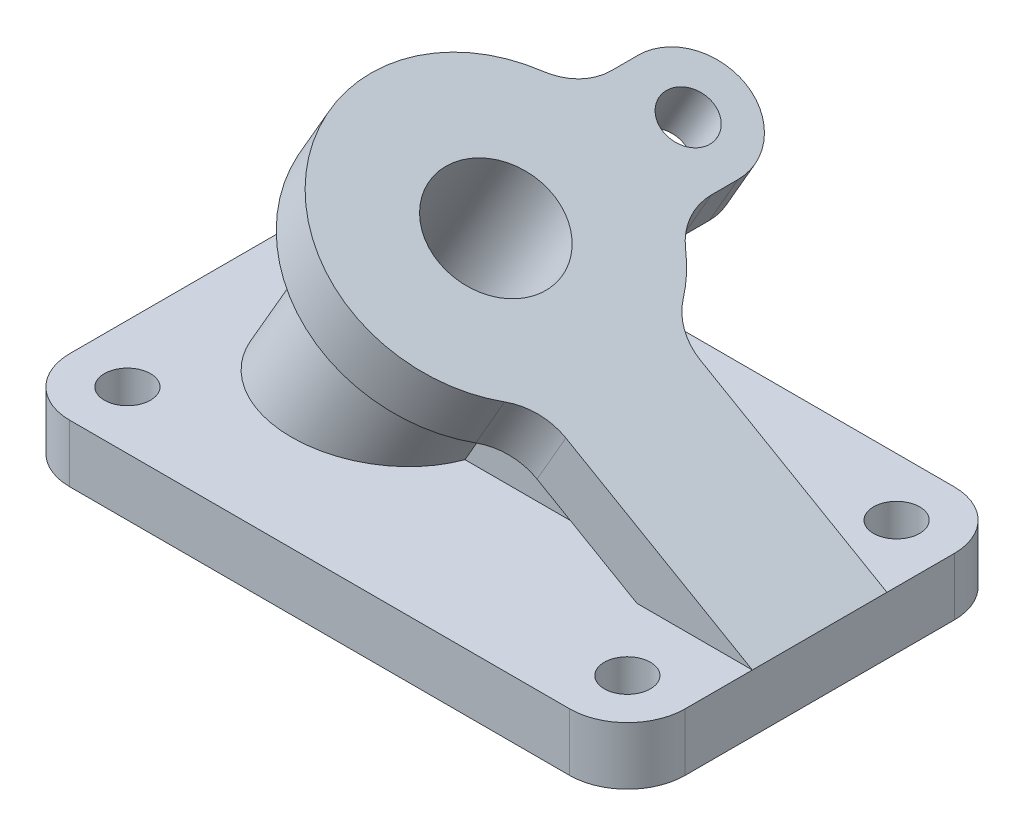
ISO-10303-21;
HEADER;
FILE_DESCRIPTION(('STEP AP214'),'2;1');
FILE_NAME('part.step','',(''),(''),'','','');
FILE_SCHEMA(('AUTOMOTIVE_DESIGN { 1 0 10303 214 1 1 1 1 }'));
ENDSEC;
DATA;
#1=APPLICATION_CONTEXT('core data for automotive mechanical design processes');
#2=APPLICATION_PROTOCOL_DEFINITION('international standard','automotive_design',2000,#1);
#3=PRODUCT_CONTEXT('',#1,'mechanical');
#4=PRODUCT('Part','Part','',(#3));
#5=PRODUCT_RELATED_PRODUCT_CATEGORY('part','',(#4));
#6=PRODUCT_DEFINITION_FORMATION('','',#4);
#7=PRODUCT_DEFINITION_CONTEXT('part definition',#1,'design');
#8=PRODUCT_DEFINITION('design','',#6,#7);
#9=PRODUCT_DEFINITION_SHAPE('','',#8);
#10=(LENGTH_UNIT() NAMED_UNIT(*) SI_UNIT(.MILLI.,.METRE.));
#11=(NAMED_UNIT(*) PLANE_ANGLE_UNIT() SI_UNIT($,.RADIAN.));
#12=(NAMED_UNIT(*) SI_UNIT($,.STERADIAN.) SOLID_ANGLE_UNIT());
#13=UNCERTAINTY_MEASURE_WITH_UNIT(LENGTH_MEASURE(1.E-05),#10,'distance_accuracy_value','');
#14=(GEOMETRIC_REPRESENTATION_CONTEXT(3) GLOBAL_UNCERTAINTY_ASSIGNED_CONTEXT((#13)) GLOBAL_UNIT_ASSIGNED_CONTEXT((#10,
#11,#12)) REPRESENTATION_CONTEXT('',''));
#15=CARTESIAN_POINT('',(0.,0.,0.));
#16=DIRECTION('',(0.,0.,1.));
#17=DIRECTION('',(1.,0.,0.));
#18=AXIS2_PLACEMENT_3D('',#15,#16,#17);
#19=CARTESIAN_POINT('',(0.,15.,0.));
#20=DIRECTION('',(0.,-1.,0.));
#21=DIRECTION('',(0.,0.,-1.));
#22=AXIS2_PLACEMENT_3D('',#19,#20,#21);
#23=PLANE('',#22);
#24=CARTESIAN_POINT('',(-65.,15.,-35.));
#25=DIRECTION('',(0.,1.,0.));
#26=DIRECTION('',(0.,0.,1.));
#27=AXIS2_PLACEMENT_3D('',#24,#25,#26);
#28=CIRCLE('',#27,6.);
#29=CARTESIAN_POINT('',(-65.,15.,-29.));
#30=VERTEX_POINT('',#29);
#31=EDGE_CURVE('E334',#30,#30,#28,.T.);
#32=ORIENTED_EDGE('',*,*,#31,.F.);
#33=EDGE_LOOP('',(#32));
#34=FACE_BOUND('',#33,.T.);
#35=CARTESIAN_POINT('',(65.,15.,-35.));
#36=DIRECTION('',(0.,1.,0.));
#37=DIRECTION('',(0.,0.,1.));
#38=AXIS2_PLACEMENT_3D('',#35,#36,#37);
#39=CIRCLE('',#38,6.);
#40=CARTESIAN_POINT('',(65.,15.,-29.));
#41=VERTEX_POINT('',#40);
#42=EDGE_CURVE('E329',#41,#41,#39,.T.);
#43=ORIENTED_EDGE('',*,*,#42,.F.);
#44=EDGE_LOOP('',(#43));
#45=FACE_BOUND('',#44,.T.);
#46=CARTESIAN_POINT('',(65.,15.,35.));
#47=DIRECTION('',(0.,1.,0.));
#48=DIRECTION('',(0.,0.,1.));
#49=AXIS2_PLACEMENT_3D('',#46,#47,#48);
#50=CIRCLE('',#49,6.);
#51=CARTESIAN_POINT('',(65.,15.,41.));
#52=VERTEX_POINT('',#51);
#53=EDGE_CURVE('E340',#52,#52,#50,.T.);
#54=ORIENTED_EDGE('',*,*,#53,.F.);
#55=EDGE_LOOP('',(#54));
#56=FACE_BOUND('',#55,.T.);
#57=CARTESIAN_POINT('',(-65.,15.,35.));
#58=DIRECTION('',(0.,1.,0.));
#59=DIRECTION('',(0.,0.,1.));
#60=AXIS2_PLACEMENT_3D('',#57,#58,#59);
#61=CIRCLE('',#60,6.);
#62=CARTESIAN_POINT('',(-65.,15.,41.));
#63=VERTEX_POINT('',#62);
#64=EDGE_CURVE('E344',#63,#63,#61,.T.);
#65=ORIENTED_EDGE('',*,*,#64,.F.);
#66=EDGE_LOOP('',(#65));
#67=FACE_BOUND('',#66,.T.);
#68=DIRECTION('',(0.,0.,1.));
#69=VECTOR('',#68,1.);
#70=CARTESIAN_POINT('',(49.9999999999997,15.,0.));
#71=LINE('',#70,#69);
#72=CARTESIAN_POINT('',(49.9999999999997,15.,-17.5));
#73=VERTEX_POINT('',#72);
#74=CARTESIAN_POINT('',(49.9999999999997,15.,-7.5));
#75=VERTEX_POINT('',#74);
#76=EDGE_CURVE('E309',#73,#75,#71,.T.);
#77=ORIENTED_EDGE('',*,*,#76,.F.);
#78=DIRECTION('',(1.,0.,0.));
#79=VECTOR('',#78,1.);
#80=CARTESIAN_POINT('',(0.,15.,-17.5));
#81=LINE('',#80,#79);
#82=CARTESIAN_POINT('',(80.,15.,-17.5));
#83=VERTEX_POINT('',#82);
#84=EDGE_CURVE('E11',#73,#83,#81,.T.);
#85=ORIENTED_EDGE('',*,*,#84,.T.);
#86=DIRECTION('',(0.,0.,-1.));
#87=VECTOR('',#86,1.);
#88=CARTESIAN_POINT('',(80.,15.,50.));
#89=LINE('',#88,#87);
#90=CARTESIAN_POINT('',(80.,15.,-35.));
#91=VERTEX_POINT('',#90);
#92=EDGE_CURVE('E360',#83,#91,#89,.T.);
#93=ORIENTED_EDGE('',*,*,#92,.T.);
#94=CARTESIAN_POINT('',(65.,15.,-35.));
#95=DIRECTION('',(0.,-1.,0.));
#96=DIRECTION('',(0.,0.,-1.));
#97=AXIS2_PLACEMENT_3D('',#94,#95,#96);
#98=CIRCLE('',#97,15.);
#99=CARTESIAN_POINT('',(65.,15.,-50.));
#100=VERTEX_POINT('',#99);
#101=EDGE_CURVE('E396',#91,#100,#98,.F.);
#102=ORIENTED_EDGE('',*,*,#101,.T.);
#103=DIRECTION('',(-1.,0.,0.));
#104=VECTOR('',#103,1.);
#105=CARTESIAN_POINT('',(-80.,15.,-50.));
#106=LINE('',#105,#104);
#107=CARTESIAN_POINT('',(-65.,15.,-50.));
#108=VERTEX_POINT('',#107);
#109=EDGE_CURVE('E357',#100,#108,#106,.T.);
#110=ORIENTED_EDGE('',*,*,#109,.T.);
#111=CARTESIAN_POINT('',(-65.,15.,-35.));
#112=DIRECTION('',(0.,-1.,0.));
#113=DIRECTION('',(0.,0.,-1.));
#114=AXIS2_PLACEMENT_3D('',#111,#112,#113);
#115=CIRCLE('',#114,15.);
#116=CARTESIAN_POINT('',(-80.,15.,-35.));
#117=VERTEX_POINT('',#116);
#118=EDGE_CURVE('E402',#108,#117,#115,.F.);
#119=ORIENTED_EDGE('',*,*,#118,.T.);
#120=DIRECTION('',(0.,0.,1.));
#121=VECTOR('',#120,1.);
#122=CARTESIAN_POINT('',(-80.,15.,50.));
#123=LINE('',#122,#121);
#124=CARTESIAN_POINT('',(-80.,15.,35.));
#125=VERTEX_POINT('',#124);
#126=EDGE_CURVE('E365',#117,#125,#123,.T.);
#127=ORIENTED_EDGE('',*,*,#126,.T.);
#128=CARTESIAN_POINT('',(-65.,15.,35.));
#129=DIRECTION('',(0.,-1.,0.));
#130=DIRECTION('',(0.,0.,-1.));
#131=AXIS2_PLACEMENT_3D('',#128,#129,#130);
#132=CIRCLE('',#131,15.);
#133=CARTESIAN_POINT('',(-65.,15.,50.));
#134=VERTEX_POINT('',#133);
#135=EDGE_CURVE('E394',#125,#134,#132,.F.);
#136=ORIENTED_EDGE('',*,*,#135,.T.);
#137=DIRECTION('',(1.,0.,0.));
#138=VECTOR('',#137,1.);
#139=CARTESIAN_POINT('',(-80.,15.,50.));
#140=LINE('',#139,#138);
#141=CARTESIAN_POINT('',(65.,15.,50.));
#142=VERTEX_POINT('',#141);
#143=EDGE_CURVE('E362',#134,#142,#140,.T.);
#144=ORIENTED_EDGE('',*,*,#143,.T.);
#145=CARTESIAN_POINT('',(65.,15.,35.));
#146=DIRECTION('',(0.,-1.,0.));
#147=DIRECTION('',(0.,0.,-1.));
#148=AXIS2_PLACEMENT_3D('',#145,#146,#147);
#149=CIRCLE('',#148,15.);
#150=CARTESIAN_POINT('',(80.,15.,35.));
#151=VERTEX_POINT('',#150);
#152=EDGE_CURVE('E400',#142,#151,#149,.F.);
#153=ORIENTED_EDGE('',*,*,#152,.T.);
#154=CARTESIAN_POINT('',(80.,15.,17.5));
#155=VERTEX_POINT('',#154);
#156=EDGE_CURVE('E351',#151,#155,#89,.T.);
#157=ORIENTED_EDGE('',*,*,#156,.T.);
#158=DIRECTION('',(1.,0.,0.));
#159=VECTOR('',#158,1.);
#160=CARTESIAN_POINT('',(0.,15.,17.5));
#161=LINE('',#160,#159);
#162=CARTESIAN_POINT('',(49.9999999999997,15.,17.5));
#163=VERTEX_POINT('',#162);
#164=EDGE_CURVE('E47',#163,#155,#161,.T.);
#165=ORIENTED_EDGE('',*,*,#164,.F.);
#166=CARTESIAN_POINT('',(49.9999999999997,15.,7.5));
#167=VERTEX_POINT('',#166);
#168=EDGE_CURVE('E308',#167,#163,#71,.T.);
#169=ORIENTED_EDGE('',*,*,#168,.F.);
#170=DIRECTION('',(1.,0.,0.));
#171=VECTOR('',#170,1.);
#172=CARTESIAN_POINT('',(-72.318551726229,15.,7.5));
#173=LINE('',#172,#171);
#174=CARTESIAN_POINT('',(-4.72434506277908,15.,7.50000000000001));
#175=VERTEX_POINT('',#174);
#176=EDGE_CURVE('E57',#175,#167,#173,.T.);
#177=ORIENTED_EDGE('',*,*,#176,.F.);
#178=CARTESIAN_POINT('',(-32.2621977992095,15.,0.));
#179=DIRECTION('',(0.,-1.,0.));
#180=DIRECTION('',(1.,0.,0.));
#181=AXIS2_PLACEMENT_3D('',#178,#179,#180);
#182=ELLIPSE('',#181,28.8675134594812,25.);
#183=CARTESIAN_POINT('',(-4.72434506277908,15.,-7.5));
#184=VERTEX_POINT('',#183);
#185=EDGE_CURVE('E322',#184,#175,#182,.F.);
#186=ORIENTED_EDGE('',*,*,#185,.F.);
#187=DIRECTION('',(-1.,0.,0.));
#188=VECTOR('',#187,1.);
#189=CARTESIAN_POINT('',(-72.318551726229,15.,-7.5));
#190=LINE('',#189,#188);
#191=EDGE_CURVE('E313',#75,#184,#190,.T.);
#192=ORIENTED_EDGE('',*,*,#191,.F.);
#193=EDGE_LOOP('',(#77,#85,#93,#102,#110,#119,#127,#136,#144,#153,#157,#165,#169,#177,#186,#192));
#194=FACE_BOUND('',#193,.T.);
#195=ADVANCED_FACE('F41',(#34,#45,#56,#67,#194),#23,.F.);
#196=CARTESIAN_POINT('',(-72.318551726229,-102.076600238408,-7.49999999999999));
#197=DIRECTION('',(0.,0.,-1.));
#198=DIRECTION('',(0.,1.,0.));
#199=AXIS2_PLACEMENT_3D('',#196,#197,#198);
#200=PLANE('',#199);
#201=DIRECTION('',(0.499999999999995,0.866025403784442,0.));
#202=VECTOR('',#201,1.);
#203=CARTESIAN_POINT('',(-72.318551726229,-102.076600238408,-7.49999999999999));
#204=LINE('',#203,#202);
#205=CARTESIAN_POINT('',(8.95674120291533,38.6963365149158,-7.5));
#206=VERTEX_POINT('',#205);
#207=EDGE_CURVE('E321',#184,#206,#204,.T.);
#208=ORIENTED_EDGE('',*,*,#207,.T.);
#209=DIRECTION('',(0.866025403784442,-0.499999999999995,0.));
#210=VECTOR('',#209,1.);
#211=CARTESIAN_POINT('',(8.95674120291531,38.6963365149158,-7.5));
#212=LINE('',#211,#210);
#213=EDGE_CURVE('E304',#206,#75,#212,.T.);
#214=ORIENTED_EDGE('',*,*,#213,.T.);
#215=ORIENTED_EDGE('',*,*,#191,.T.);
#216=EDGE_LOOP('',(#208,#214,#215));
#217=FACE_BOUND('',#216,.T.);
#218=ADVANCED_FACE('F496',(#217),#200,.T.);
#219=CARTESIAN_POINT('',(-92.971941278552,-90.152360220696,0.));
#220=DIRECTION('',(0.499999999999995,0.866025403784442,0.));
#221=DIRECTION('',(-0.866025403784442,0.499999999999995,0.));
#222=AXIS2_PLACEMENT_3D('',#219,#220,#221);
#223=CYLINDRICAL_SURFACE('',#222,25.);
#224=DIRECTION('',(0.499999999999995,0.866025403784442,0.));
#225=VECTOR('',#224,1.);
#226=CARTESIAN_POINT('',(-72.318551726229,-102.076600238408,7.50000000000001));
#227=LINE('',#226,#225);
#228=CARTESIAN_POINT('',(8.95674120291534,38.6963365149158,7.50000000000001));
#229=VERTEX_POINT('',#228);
#230=EDGE_CURVE('E318',#175,#229,#227,.T.);
#231=ORIENTED_EDGE('',*,*,#230,.T.);
#232=CARTESIAN_POINT('',(-11.6966483494076,50.6205765326275,0.));
#233=DIRECTION('',(0.499999999999995,0.866025403784442,0.));
#234=DIRECTION('',(-0.866025403784442,0.499999999999995,0.));
#235=AXIS2_PLACEMENT_3D('',#232,#233,#234);
#236=CIRCLE('',#235,25.);
#237=EDGE_CURVE('E284',#229,#206,#236,.F.);
#238=ORIENTED_EDGE('',*,*,#237,.T.);
#239=ORIENTED_EDGE('',*,*,#207,.F.);
#240=ORIENTED_EDGE('',*,*,#185,.T.);
#241=EDGE_LOOP('',(#231,#238,#239,#240));
#242=FACE_BOUND('',#241,.T.);
#243=ADVANCED_FACE('F494',(#242),#223,.T.);
#244=CARTESIAN_POINT('',(-72.318551726229,-102.076600238408,7.50000000000001));
#245=DIRECTION('',(0.,0.,1.));
#246=DIRECTION('',(0.,-1.,0.));
#247=AXIS2_PLACEMENT_3D('',#244,#245,#246);
#248=PLANE('',#247);
#249=ORIENTED_EDGE('',*,*,#176,.T.);
#250=DIRECTION('',(-0.866025403784442,0.499999999999995,0.));
#251=VECTOR('',#250,1.);
#252=CARTESIAN_POINT('',(8.95674120291531,38.6963365149158,7.5));
#253=LINE('',#252,#251);
#254=EDGE_CURVE('E412',#167,#229,#253,.T.);
#255=ORIENTED_EDGE('',*,*,#254,.T.);
#256=ORIENTED_EDGE('',*,*,#230,.F.);
#257=EDGE_LOOP('',(#249,#255,#256));
#258=FACE_BOUND('',#257,.T.);
#259=ADVANCED_FACE('F493',(#258),#248,.T.);
#260=CARTESIAN_POINT('',(80.,15.,50.));
#261=DIRECTION('',(-1.,0.,0.));
#262=DIRECTION('',(0.,0.,1.));
#263=AXIS2_PLACEMENT_3D('',#260,#261,#262);
#264=PLANE('',#263);
#265=DIRECTION('',(0.,0.,-1.));
#266=VECTOR('',#265,1.);
#267=CARTESIAN_POINT('',(80.,0.,50.));
#268=LINE('',#267,#266);
#269=CARTESIAN_POINT('',(80.,0.,35.));
#270=VERTEX_POINT('',#269);
#271=CARTESIAN_POINT('',(80.,0.,-35.));
#272=VERTEX_POINT('',#271);
#273=EDGE_CURVE('E352',#270,#272,#268,.T.);
#274=ORIENTED_EDGE('',*,*,#273,.T.);
#275=DIRECTION('',(0.,-1.,0.));
#276=VECTOR('',#275,1.);
#277=CARTESIAN_POINT('',(80.,15.,-35.));
#278=LINE('',#277,#276);
#279=EDGE_CURVE('E407',#272,#91,#278,.F.);
#280=ORIENTED_EDGE('',*,*,#279,.T.);
#281=ORIENTED_EDGE('',*,*,#92,.F.);
#282=EDGE_CURVE('E356',#155,#83,#89,.T.);
#283=ORIENTED_EDGE('',*,*,#282,.F.);
#284=ORIENTED_EDGE('',*,*,#156,.F.);
#285=DIRECTION('',(0.,-1.,0.));
#286=VECTOR('',#285,1.);
#287=CARTESIAN_POINT('',(80.,15.,35.));
#288=LINE('',#287,#286);
#289=EDGE_CURVE('E401',#151,#270,#288,.T.);
#290=ORIENTED_EDGE('',*,*,#289,.T.);
#291=EDGE_LOOP('',(#274,#280,#281,#283,#284,#290));
#292=FACE_BOUND('',#291,.T.);
#293=ADVANCED_FACE('F431',(#292),#264,.F.);
#294=CARTESIAN_POINT('',(-80.,15.,-50.));
#295=DIRECTION('',(0.,0.,1.));
#296=DIRECTION('',(1.,0.,0.));
#297=AXIS2_PLACEMENT_3D('',#294,#295,#296);
#298=PLANE('',#297);
#299=DIRECTION('',(-1.,0.,0.));
#300=VECTOR('',#299,1.);
#301=CARTESIAN_POINT('',(-80.,0.,-50.));
#302=LINE('',#301,#300);
#303=CARTESIAN_POINT('',(65.,0.,-50.));
#304=VERTEX_POINT('',#303);
#305=CARTESIAN_POINT('',(-65.,0.,-50.));
#306=VERTEX_POINT('',#305);
#307=EDGE_CURVE('E369',#304,#306,#302,.T.);
#308=ORIENTED_EDGE('',*,*,#307,.T.);
#309=DIRECTION('',(0.,-1.,0.));
#310=VECTOR('',#309,1.);
#311=CARTESIAN_POINT('',(-65.,15.,-50.));
#312=LINE('',#311,#310);
#313=EDGE_CURVE('E392',#306,#108,#312,.F.);
#314=ORIENTED_EDGE('',*,*,#313,.T.);
#315=ORIENTED_EDGE('',*,*,#109,.F.);
#316=DIRECTION('',(0.,-1.,0.));
#317=VECTOR('',#316,1.);
#318=CARTESIAN_POINT('',(65.,15.,-50.));
#319=LINE('',#318,#317);
#320=EDGE_CURVE('E388',#100,#304,#319,.T.);
#321=ORIENTED_EDGE('',*,*,#320,.T.);
#322=EDGE_LOOP('',(#308,#314,#315,#321));
#323=FACE_BOUND('',#322,.T.);
#324=ADVANCED_FACE('F453',(#323),#298,.F.);
#325=CARTESIAN_POINT('',(-80.,15.,50.));
#326=DIRECTION('',(1.,0.,0.));
#327=DIRECTION('',(0.,0.,-1.));
#328=AXIS2_PLACEMENT_3D('',#325,#326,#327);
#329=PLANE('',#328);
#330=ORIENTED_EDGE('',*,*,#126,.F.);
#331=DIRECTION('',(0.,-1.,0.));
#332=VECTOR('',#331,1.);
#333=CARTESIAN_POINT('',(-80.,15.,-35.));
#334=LINE('',#333,#332);
#335=CARTESIAN_POINT('',(-80.,0.,-35.));
#336=VERTEX_POINT('',#335);
#337=EDGE_CURVE('E378',#117,#336,#334,.T.);
#338=ORIENTED_EDGE('',*,*,#337,.T.);
#339=DIRECTION('',(0.,0.,1.));
#340=VECTOR('',#339,1.);
#341=CARTESIAN_POINT('',(-80.,0.,50.));
#342=LINE('',#341,#340);
#343=CARTESIAN_POINT('',(-80.,0.,35.));
#344=VERTEX_POINT('',#343);
#345=EDGE_CURVE('E373',#336,#344,#342,.T.);
#346=ORIENTED_EDGE('',*,*,#345,.T.);
#347=DIRECTION('',(0.,-1.,0.));
#348=VECTOR('',#347,1.);
#349=CARTESIAN_POINT('',(-80.,15.,35.));
#350=LINE('',#349,#348);
#351=EDGE_CURVE('E370',#344,#125,#350,.F.);
#352=ORIENTED_EDGE('',*,*,#351,.T.);
#353=EDGE_LOOP('',(#330,#338,#346,#352));
#354=FACE_BOUND('',#353,.T.);
#355=ADVANCED_FACE('F450',(#354),#329,.F.);
#356=CARTESIAN_POINT('',(-80.,15.,50.));
#357=DIRECTION('',(0.,0.,-1.));
#358=DIRECTION('',(-1.,0.,0.));
#359=AXIS2_PLACEMENT_3D('',#356,#357,#358);
#360=PLANE('',#359);
#361=DIRECTION('',(1.,0.,0.));
#362=VECTOR('',#361,1.);
#363=CARTESIAN_POINT('',(-80.,0.,50.));
#364=LINE('',#363,#362);
#365=CARTESIAN_POINT('',(-65.,0.,50.));
#366=VERTEX_POINT('',#365);
#367=CARTESIAN_POINT('',(65.,0.,50.));
#368=VERTEX_POINT('',#367);
#369=EDGE_CURVE('E376',#366,#368,#364,.T.);
#370=ORIENTED_EDGE('',*,*,#369,.T.);
#371=DIRECTION('',(0.,-1.,0.));
#372=VECTOR('',#371,1.);
#373=CARTESIAN_POINT('',(65.,15.,50.));
#374=LINE('',#373,#372);
#375=EDGE_CURVE('E61',#368,#142,#374,.F.);
#376=ORIENTED_EDGE('',*,*,#375,.T.);
#377=ORIENTED_EDGE('',*,*,#143,.F.);
#378=DIRECTION('',(0.,-1.,0.));
#379=VECTOR('',#378,1.);
#380=CARTESIAN_POINT('',(-65.,15.,50.));
#381=LINE('',#380,#379);
#382=EDGE_CURVE('E406',#134,#366,#381,.T.);
#383=ORIENTED_EDGE('',*,*,#382,.T.);
#384=EDGE_LOOP('',(#370,#376,#377,#383));
#385=FACE_BOUND('',#384,.T.);
#386=ADVANCED_FACE('F439',(#385),#360,.F.);
#387=CARTESIAN_POINT('',(0.,0.,0.));
#388=DIRECTION('',(0.,-1.,0.));
#389=DIRECTION('',(0.,0.,-1.));
#390=AXIS2_PLACEMENT_3D('',#387,#388,#389);
#391=PLANE('',#390);
#392=CARTESIAN_POINT('',(-65.,0.,35.));
#393=DIRECTION('',(0.,1.,0.));
#394=DIRECTION('',(0.,0.,1.));
#395=AXIS2_PLACEMENT_3D('',#392,#393,#394);
#396=CIRCLE('',#395,6.);
#397=CARTESIAN_POINT('',(-65.,0.,41.));
#398=VERTEX_POINT('',#397);
#399=EDGE_CURVE('E316',#398,#398,#396,.T.);
#400=ORIENTED_EDGE('',*,*,#399,.T.);
#401=EDGE_LOOP('',(#400));
#402=FACE_BOUND('',#401,.T.);
#403=CARTESIAN_POINT('',(65.,0.,35.));
#404=DIRECTION('',(0.,1.,0.));
#405=DIRECTION('',(0.,0.,1.));
#406=AXIS2_PLACEMENT_3D('',#403,#404,#405);
#407=CIRCLE('',#406,6.);
#408=CARTESIAN_POINT('',(65.,0.,41.));
#409=VERTEX_POINT('',#408);
#410=EDGE_CURVE('E338',#409,#409,#407,.T.);
#411=ORIENTED_EDGE('',*,*,#410,.T.);
#412=EDGE_LOOP('',(#411));
#413=FACE_BOUND('',#412,.T.);
#414=CARTESIAN_POINT('',(65.,0.,-35.));
#415=DIRECTION('',(0.,1.,0.));
#416=DIRECTION('',(0.,0.,1.));
#417=AXIS2_PLACEMENT_3D('',#414,#415,#416);
#418=CIRCLE('',#417,6.);
#419=CARTESIAN_POINT('',(65.,0.,-29.));
#420=VERTEX_POINT('',#419);
#421=EDGE_CURVE('E331',#420,#420,#418,.T.);
#422=ORIENTED_EDGE('',*,*,#421,.T.);
#423=EDGE_LOOP('',(#422));
#424=FACE_BOUND('',#423,.T.);
#425=CARTESIAN_POINT('',(-65.,0.,-35.));
#426=DIRECTION('',(0.,1.,0.));
#427=DIRECTION('',(0.,0.,1.));
#428=AXIS2_PLACEMENT_3D('',#425,#426,#427);
#429=CIRCLE('',#428,6.);
#430=CARTESIAN_POINT('',(-65.,0.,-29.));
#431=VERTEX_POINT('',#430);
#432=EDGE_CURVE('E347',#431,#431,#429,.T.);
#433=ORIENTED_EDGE('',*,*,#432,.T.);
#434=EDGE_LOOP('',(#433));
#435=FACE_BOUND('',#434,.T.);
#436=ORIENTED_EDGE('',*,*,#345,.F.);
#437=CARTESIAN_POINT('',(-65.,0.,-35.));
#438=DIRECTION('',(0.,-1.,0.));
#439=DIRECTION('',(0.,0.,-1.));
#440=AXIS2_PLACEMENT_3D('',#437,#438,#439);
#441=CIRCLE('',#440,15.);
#442=EDGE_CURVE('E389',#336,#306,#441,.T.);
#443=ORIENTED_EDGE('',*,*,#442,.T.);
#444=ORIENTED_EDGE('',*,*,#307,.F.);
#445=CARTESIAN_POINT('',(65.,0.,-35.));
#446=DIRECTION('',(0.,-1.,0.));
#447=DIRECTION('',(0.,0.,-1.));
#448=AXIS2_PLACEMENT_3D('',#445,#446,#447);
#449=CIRCLE('',#448,15.);
#450=EDGE_CURVE('E387',#304,#272,#449,.T.);
#451=ORIENTED_EDGE('',*,*,#450,.T.);
#452=ORIENTED_EDGE('',*,*,#273,.F.);
#453=CARTESIAN_POINT('',(65.,0.,35.));
#454=DIRECTION('',(0.,-1.,0.));
#455=DIRECTION('',(0.,0.,-1.));
#456=AXIS2_PLACEMENT_3D('',#453,#454,#455);
#457=CIRCLE('',#456,15.);
#458=EDGE_CURVE('E381',#270,#368,#457,.T.);
#459=ORIENTED_EDGE('',*,*,#458,.T.);
#460=ORIENTED_EDGE('',*,*,#369,.F.);
#461=CARTESIAN_POINT('',(-65.,0.,35.));
#462=DIRECTION('',(0.,-1.,0.));
#463=DIRECTION('',(0.,0.,-1.));
#464=AXIS2_PLACEMENT_3D('',#461,#462,#463);
#465=CIRCLE('',#464,15.);
#466=EDGE_CURVE('E385',#366,#344,#465,.T.);
#467=ORIENTED_EDGE('',*,*,#466,.T.);
#468=EDGE_LOOP('',(#436,#443,#444,#451,#452,#459,#460,#467));
#469=FACE_BOUND('',#468,.T.);
#470=ADVANCED_FACE('F437',(#402,#413,#424,#435,#469),#391,.T.);
#471=CARTESIAN_POINT('',(-65.,15.,-35.));
#472=DIRECTION('',(0.,-1.,0.));
#473=DIRECTION('',(0.,0.,-1.));
#474=AXIS2_PLACEMENT_3D('',#471,#472,#473);
#475=CYLINDRICAL_SURFACE('',#474,15.);
#476=ORIENTED_EDGE('',*,*,#118,.F.);
#477=ORIENTED_EDGE('',*,*,#313,.F.);
#478=ORIENTED_EDGE('',*,*,#442,.F.);
#479=ORIENTED_EDGE('',*,*,#337,.F.);
#480=EDGE_LOOP('',(#476,#477,#478,#479));
#481=FACE_BOUND('',#480,.T.);
#482=ADVANCED_FACE('F452',(#481),#475,.T.);
#483=CARTESIAN_POINT('',(65.,15.,-35.));
#484=DIRECTION('',(0.,-1.,0.));
#485=DIRECTION('',(0.,0.,-1.));
#486=AXIS2_PLACEMENT_3D('',#483,#484,#485);
#487=CYLINDRICAL_SURFACE('',#486,15.);
#488=ORIENTED_EDGE('',*,*,#101,.F.);
#489=ORIENTED_EDGE('',*,*,#279,.F.);
#490=ORIENTED_EDGE('',*,*,#450,.F.);
#491=ORIENTED_EDGE('',*,*,#320,.F.);
#492=EDGE_LOOP('',(#488,#489,#490,#491));
#493=FACE_BOUND('',#492,.T.);
#494=ADVANCED_FACE('F459',(#493),#487,.T.);
#495=CARTESIAN_POINT('',(65.,15.,35.));
#496=DIRECTION('',(0.,-1.,0.));
#497=DIRECTION('',(0.,0.,-1.));
#498=AXIS2_PLACEMENT_3D('',#495,#496,#497);
#499=CYLINDRICAL_SURFACE('',#498,15.);
#500=ORIENTED_EDGE('',*,*,#152,.F.);
#501=ORIENTED_EDGE('',*,*,#375,.F.);
#502=ORIENTED_EDGE('',*,*,#458,.F.);
#503=ORIENTED_EDGE('',*,*,#289,.F.);
#504=EDGE_LOOP('',(#500,#501,#502,#503));
#505=FACE_BOUND('',#504,.T.);
#506=ADVANCED_FACE('F434',(#505),#499,.T.);
#507=CARTESIAN_POINT('',(-65.,15.,35.));
#508=DIRECTION('',(0.,-1.,0.));
#509=DIRECTION('',(0.,0.,-1.));
#510=AXIS2_PLACEMENT_3D('',#507,#508,#509);
#511=CYLINDRICAL_SURFACE('',#510,15.);
#512=ORIENTED_EDGE('',*,*,#135,.F.);
#513=ORIENTED_EDGE('',*,*,#351,.F.);
#514=ORIENTED_EDGE('',*,*,#466,.F.);
#515=ORIENTED_EDGE('',*,*,#382,.F.);
#516=EDGE_LOOP('',(#512,#513,#514,#515));
#517=FACE_BOUND('',#516,.T.);
#518=ADVANCED_FACE('F43',(#517),#511,.T.);
#519=CARTESIAN_POINT('',(-65.,0.,-35.));
#520=DIRECTION('',(0.,1.,0.));
#521=DIRECTION('',(0.,0.,1.));
#522=AXIS2_PLACEMENT_3D('',#519,#520,#521);
#523=CYLINDRICAL_SURFACE('',#522,6.);
#524=ORIENTED_EDGE('',*,*,#432,.F.);
#525=EDGE_LOOP('',(#524));
#526=FACE_BOUND('',#525,.T.);
#527=ORIENTED_EDGE('',*,*,#31,.T.);
#528=EDGE_LOOP('',(#527));
#529=FACE_BOUND('',#528,.T.);
#530=ADVANCED_FACE('F519',(#526,#529),#523,.F.);
#531=CARTESIAN_POINT('',(65.,0.,-35.));
#532=DIRECTION('',(0.,1.,0.));
#533=DIRECTION('',(0.,0.,1.));
#534=AXIS2_PLACEMENT_3D('',#531,#532,#533);
#535=CYLINDRICAL_SURFACE('',#534,6.);
#536=ORIENTED_EDGE('',*,*,#421,.F.);
#537=EDGE_LOOP('',(#536));
#538=FACE_BOUND('',#537,.T.);
#539=ORIENTED_EDGE('',*,*,#42,.T.);
#540=EDGE_LOOP('',(#539));
#541=FACE_BOUND('',#540,.T.);
#542=ADVANCED_FACE('F511',(#538,#541),#535,.F.);
#543=CARTESIAN_POINT('',(65.,0.,35.));
#544=DIRECTION('',(0.,1.,0.));
#545=DIRECTION('',(0.,0.,1.));
#546=AXIS2_PLACEMENT_3D('',#543,#544,#545);
#547=CYLINDRICAL_SURFACE('',#546,6.);
#548=ORIENTED_EDGE('',*,*,#410,.F.);
#549=EDGE_LOOP('',(#548));
#550=FACE_BOUND('',#549,.T.);
#551=ORIENTED_EDGE('',*,*,#53,.T.);
#552=EDGE_LOOP('',(#551));
#553=FACE_BOUND('',#552,.T.);
#554=ADVANCED_FACE('F520',(#550,#553),#547,.F.);
#555=CARTESIAN_POINT('',(-65.,0.,35.));
#556=DIRECTION('',(0.,1.,0.));
#557=DIRECTION('',(0.,0.,1.));
#558=AXIS2_PLACEMENT_3D('',#555,#556,#557);
#559=CYLINDRICAL_SURFACE('',#558,6.);
#560=ORIENTED_EDGE('',*,*,#399,.F.);
#561=EDGE_LOOP('',(#560));
#562=FACE_BOUND('',#561,.T.);
#563=ORIENTED_EDGE('',*,*,#64,.T.);
#564=EDGE_LOOP('',(#563));
#565=FACE_BOUND('',#564,.T.);
#566=ADVANCED_FACE('F515',(#562,#565),#559,.F.);
#567=CARTESIAN_POINT('',(-92.971941278552,-90.152360220696,0.));
#568=DIRECTION('',(0.499999999999995,0.866025403784442,0.));
#569=DIRECTION('',(-0.866025403784442,0.499999999999995,0.));
#570=AXIS2_PLACEMENT_3D('',#567,#568,#569);
#571=CYLINDRICAL_SURFACE('',#570,15.);
#572=CARTESIAN_POINT('',(-4.19664834940771,63.6109575893941,0.));
#573=DIRECTION('',(0.499999999999995,0.866025403784442,0.));
#574=DIRECTION('',(-0.866025403784442,0.499999999999995,0.));
#575=AXIS2_PLACEMENT_3D('',#572,#573,#574);
#576=CIRCLE('',#575,15.);
#577=CARTESIAN_POINT('',(-17.1870294061743,71.110957589394,0.));
#578=VERTEX_POINT('',#577);
#579=EDGE_CURVE('E311',#578,#578,#576,.T.);
#580=ORIENTED_EDGE('',*,*,#579,.T.);
#581=EDGE_LOOP('',(#580));
#582=FACE_BOUND('',#581,.T.);
#583=CARTESIAN_POINT('',(-32.2621977992095,15.,0.));
#584=DIRECTION('',(0.,-1.,0.));
#585=DIRECTION('',(1.,0.,0.));
#586=AXIS2_PLACEMENT_3D('',#583,#584,#585);
#587=ELLIPSE('',#586,17.3205080756887,15.);
#588=CARTESIAN_POINT('',(-14.9416897235208,15.,0.));
#589=VERTEX_POINT('',#588);
#590=EDGE_CURVE('E314',#589,#589,#587,.F.);
#591=ORIENTED_EDGE('',*,*,#590,.F.);
#592=EDGE_LOOP('',(#591));
#593=FACE_BOUND('',#592,.T.);
#594=ADVANCED_FACE('F508',(#582,#593),#571,.F.);
#595=CARTESIAN_POINT('',(-4.19664834940771,63.6109575893941,0.));
#596=DIRECTION('',(0.499999999999995,0.866025403784442,0.));
#597=DIRECTION('',(-0.866025403784442,0.499999999999995,0.));
#598=AXIS2_PLACEMENT_3D('',#595,#596,#597);
#599=PLANE('',#598);
#600=ORIENTED_EDGE('',*,*,#579,.F.);
#601=EDGE_LOOP('',(#600));
#602=FACE_BOUND('',#601,.T.);
#603=DIRECTION('',(-0.866025403784442,0.499999999999995,0.));
#604=VECTOR('',#603,1.);
#605=CARTESIAN_POINT('',(26.4951905283828,45.8910161513774,17.5));
#606=LINE('',#605,#604);
#607=CARTESIAN_POINT('',(31.5104937933067,42.995429461306,17.5));
#608=VERTEX_POINT('',#607);
#609=EDGE_CURVE('E277',#155,#608,#606,.T.);
#610=ORIENTED_EDGE('',*,*,#609,.F.);
#611=ORIENTED_EDGE('',*,*,#282,.T.);
#612=DIRECTION('',(-0.866025403784442,0.499999999999995,0.));
#613=VECTOR('',#612,1.);
#614=CARTESIAN_POINT('',(26.4951905283828,45.8910161513774,-17.5));
#615=LINE('',#614,#613);
#616=CARTESIAN_POINT('',(31.5104937933067,42.995429461306,-17.5));
#617=VERTEX_POINT('',#616);
#618=EDGE_CURVE('E276',#83,#617,#615,.T.);
#619=ORIENTED_EDGE('',*,*,#618,.T.);
#620=CARTESIAN_POINT('',(31.5104937933067,42.995429461306,-32.5));
#621=DIRECTION('',(0.499999999999995,0.866025403784442,0.));
#622=DIRECTION('',(-0.866025403784442,0.499999999999995,0.));
#623=AXIS2_PLACEMENT_3D('',#620,#621,#622);
#624=CIRCLE('',#623,15.);
#625=CARTESIAN_POINT('',(21.3084531811025,48.8855803550455,-23.2142857142857));
#626=VERTEX_POINT('',#625);
#627=EDGE_CURVE('E229',#617,#626,#624,.F.);
#628=ORIENTED_EDGE('',*,*,#627,.T.);
#629=CARTESIAN_POINT('',(-4.1966483494077,63.6109575893941,0.));
#630=DIRECTION('',(0.499999999999995,0.866025403784442,0.));
#631=DIRECTION('',(-0.866025403784442,0.499999999999995,0.));
#632=AXIS2_PLACEMENT_3D('',#629,#630,#631);
#633=CIRCLE('',#632,37.5);
#634=CARTESIAN_POINT('',(14.3610388745446,52.8966718751085,-30.7744427493109));
#635=VERTEX_POINT('',#634);
#636=EDGE_CURVE('E253',#626,#635,#633,.T.);
#637=ORIENTED_EDGE('',*,*,#636,.T.);
#638=CARTESIAN_POINT('',(21.7841137641256,48.6109575893943,-43.0842198490352));
#639=DIRECTION('',(0.499999999999995,0.866025403784442,0.));
#640=DIRECTION('',(-0.866025403784442,0.499999999999995,0.));
#641=AXIS2_PLACEMENT_3D('',#638,#639,#640);
#642=CIRCLE('',#641,15.);
#643=CARTESIAN_POINT('',(8.79373270735892,56.1109575893942,-43.0842198490352));
#644=VERTEX_POINT('',#643);
#645=EDGE_CURVE('E203',#635,#644,#642,.F.);
#646=ORIENTED_EDGE('',*,*,#645,.T.);
#647=DIRECTION('',(0.,0.,-1.));
#648=VECTOR('',#647,1.);
#649=CARTESIAN_POINT('',(8.79373270735892,56.1109575893942,0.));
#650=LINE('',#649,#648);
#651=CARTESIAN_POINT('',(8.79373270735892,56.1109575893942,-50.));
#652=VERTEX_POINT('',#651);
#653=EDGE_CURVE('E259',#644,#652,#650,.T.);
#654=ORIENTED_EDGE('',*,*,#653,.T.);
#655=CARTESIAN_POINT('',(-4.1966483494077,63.6109575893941,-50.));
#656=DIRECTION('',(0.499999999999995,0.866025403784442,0.));
#657=DIRECTION('',(-0.866025403784442,0.499999999999995,0.));
#658=AXIS2_PLACEMENT_3D('',#655,#656,#657);
#659=CIRCLE('',#658,15.);
#660=CARTESIAN_POINT('',(-17.1870294061743,71.110957589394,-50.));
#661=VERTEX_POINT('',#660);
#662=EDGE_CURVE('E261',#652,#661,#659,.T.);
#663=ORIENTED_EDGE('',*,*,#662,.T.);
#664=DIRECTION('',(0.,0.,-1.));
#665=VECTOR('',#664,1.);
#666=CARTESIAN_POINT('',(-17.1870294061743,71.110957589394,0.));
#667=LINE('',#666,#665);
#668=CARTESIAN_POINT('',(-17.1870294061743,71.110957589394,-43.0842198490352));
#669=VERTEX_POINT('',#668);
#670=EDGE_CURVE('E263',#669,#661,#667,.T.);
#671=ORIENTED_EDGE('',*,*,#670,.F.);
#672=CARTESIAN_POINT('',(-30.1774104629409,78.6109575893939,-43.0842198490352));
#673=DIRECTION('',(0.499999999999995,0.866025403784442,0.));
#674=DIRECTION('',(-0.866025403784442,0.499999999999995,0.));
#675=AXIS2_PLACEMENT_3D('',#672,#673,#674);
#676=CIRCLE('',#675,15.);
#677=CARTESIAN_POINT('',(-22.75433557336,74.3252433036797,-30.7744427493109));
#678=VERTEX_POINT('',#677);
#679=EDGE_CURVE('E270',#678,#669,#676,.T.);
#680=ORIENTED_EDGE('',*,*,#679,.F.);
#681=CARTESIAN_POINT('',(-4.1966483494077,63.6109575893941,0.));
#682=DIRECTION('',(0.499999999999995,0.866025403784442,0.));
#683=DIRECTION('',(-0.866025403784442,0.499999999999995,0.));
#684=AXIS2_PLACEMENT_3D('',#681,#682,#683);
#685=CIRCLE('',#684,37.5);
#686=CARTESIAN_POINT('',(21.3084531811025,48.8855803550455,23.2142857142857));
#687=VERTEX_POINT('',#686);
#688=EDGE_CURVE('E268',#678,#687,#685,.T.);
#689=ORIENTED_EDGE('',*,*,#688,.T.);
#690=CARTESIAN_POINT('',(31.5104937933067,42.995429461306,32.5));
#691=DIRECTION('',(0.499999999999995,0.866025403784442,0.));
#692=DIRECTION('',(-0.866025403784442,0.499999999999995,0.));
#693=AXIS2_PLACEMENT_3D('',#690,#691,#692);
#694=CIRCLE('',#693,15.);
#695=EDGE_CURVE('E271',#608,#687,#694,.T.);
#696=ORIENTED_EDGE('',*,*,#695,.F.);
#697=EDGE_LOOP('',(#610,#611,#619,#628,#637,#646,#654,#663,#671,#680,#689,#696));
#698=FACE_BOUND('',#697,.T.);
#699=CARTESIAN_POINT('',(-4.1966483494077,63.6109575893941,-50.));
#700=DIRECTION('',(0.499999999999995,0.866025403784442,0.));
#701=DIRECTION('',(-0.866025403784442,0.499999999999995,0.));
#702=AXIS2_PLACEMENT_3D('',#699,#700,#701);
#703=CIRCLE('',#702,6.50000000000001);
#704=CARTESIAN_POINT('',(-9.82581347400658,66.8609575893941,-50.));
#705=VERTEX_POINT('',#704);
#706=EDGE_CURVE('E255',#705,#705,#703,.T.);
#707=ORIENTED_EDGE('',*,*,#706,.F.);
#708=EDGE_LOOP('',(#707));
#709=FACE_BOUND('',#708,.T.);
#710=ADVANCED_FACE('F421',(#602,#698,#709),#599,.T.);
#711=ORIENTED_EDGE('',*,*,#590,.T.);
#712=EDGE_LOOP('',(#711));
#713=FACE_BOUND('',#712,.T.);
#714=ADVANCED_FACE('F506',(#713),#23,.F.);
#715=CARTESIAN_POINT('',(18.9951905283829,32.9006350946107,-17.5));
#716=DIRECTION('',(0.,0.,-1.));
#717=DIRECTION('',(-1.,0.,0.));
#718=AXIS2_PLACEMENT_3D('',#715,#716,#717);
#719=PLANE('',#718);
#720=ORIENTED_EDGE('',*,*,#84,.F.);
#721=DIRECTION('',(-0.866025403784442,0.499999999999995,0.));
#722=VECTOR('',#721,1.);
#723=CARTESIAN_POINT('',(18.9951905283829,32.9006350946107,-17.5));
#724=LINE('',#723,#722);
#725=CARTESIAN_POINT('',(24.0104937933067,30.0050484045394,-17.5));
#726=VERTEX_POINT('',#725);
#727=EDGE_CURVE('E248',#73,#726,#724,.T.);
#728=ORIENTED_EDGE('',*,*,#727,.T.);
#729=DIRECTION('',(0.499999999999995,0.866025403784442,0.));
#730=VECTOR('',#729,1.);
#731=CARTESIAN_POINT('',(24.0104937933067,30.0050484045394,-17.5));
#732=LINE('',#731,#730);
#733=EDGE_CURVE('E287',#726,#617,#732,.T.);
#734=ORIENTED_EDGE('',*,*,#733,.T.);
#735=ORIENTED_EDGE('',*,*,#618,.F.);
#736=EDGE_LOOP('',(#720,#728,#734,#735));
#737=FACE_BOUND('',#736,.T.);
#738=ADVANCED_FACE('F461',(#737),#719,.T.);
#739=CARTESIAN_POINT('',(18.9951905283829,32.9006350946107,17.5));
#740=DIRECTION('',(0.,0.,-1.));
#741=DIRECTION('',(-1.,0.,0.));
#742=AXIS2_PLACEMENT_3D('',#739,#740,#741);
#743=PLANE('',#742);
#744=DIRECTION('',(-0.866025403784442,0.499999999999995,0.));
#745=VECTOR('',#744,1.);
#746=CARTESIAN_POINT('',(18.9951905283829,32.9006350946107,17.5));
#747=LINE('',#746,#745);
#748=CARTESIAN_POINT('',(24.0104937933067,30.0050484045394,17.5));
#749=VERTEX_POINT('',#748);
#750=EDGE_CURVE('E250',#163,#749,#747,.T.);
#751=ORIENTED_EDGE('',*,*,#750,.F.);
#752=ORIENTED_EDGE('',*,*,#164,.T.);
#753=ORIENTED_EDGE('',*,*,#609,.T.);
#754=DIRECTION('',(0.499999999999995,0.866025403784442,0.));
#755=VECTOR('',#754,1.);
#756=CARTESIAN_POINT('',(24.0104937933067,30.0050484045394,17.5));
#757=LINE('',#756,#755);
#758=EDGE_CURVE('E289',#749,#608,#757,.T.);
#759=ORIENTED_EDGE('',*,*,#758,.F.);
#760=EDGE_LOOP('',(#751,#752,#753,#759));
#761=FACE_BOUND('',#760,.T.);
#762=ADVANCED_FACE('F418',(#761),#743,.F.);
#763=CARTESIAN_POINT('',(18.9951905283829,32.9006350946107,0.));
#764=DIRECTION('',(0.499999999999995,0.866025403784442,0.));
#765=DIRECTION('',(-0.866025403784442,0.499999999999995,0.));
#766=AXIS2_PLACEMENT_3D('',#763,#764,#765);
#767=PLANE('',#766);
#768=CARTESIAN_POINT('',(-11.6966483494076,50.6205765326275,-50.));
#769=DIRECTION('',(0.499999999999995,0.866025403784442,0.));
#770=DIRECTION('',(-0.866025403784442,0.499999999999995,0.));
#771=AXIS2_PLACEMENT_3D('',#768,#769,#770);
#772=CIRCLE('',#771,6.50000000000001);
#773=CARTESIAN_POINT('',(-17.3258134740065,53.8705765326274,-50.));
#774=VERTEX_POINT('',#773);
#775=EDGE_CURVE('E227',#774,#774,#772,.T.);
#776=ORIENTED_EDGE('',*,*,#775,.T.);
#777=EDGE_LOOP('',(#776));
#778=FACE_BOUND('',#777,.T.);
#779=ORIENTED_EDGE('',*,*,#727,.F.);
#780=ORIENTED_EDGE('',*,*,#76,.T.);
#781=ORIENTED_EDGE('',*,*,#213,.F.);
#782=ORIENTED_EDGE('',*,*,#237,.F.);
#783=ORIENTED_EDGE('',*,*,#254,.F.);
#784=ORIENTED_EDGE('',*,*,#168,.T.);
#785=ORIENTED_EDGE('',*,*,#750,.T.);
#786=CARTESIAN_POINT('',(24.0104937933067,30.0050484045394,32.5));
#787=DIRECTION('',(0.499999999999995,0.866025403784442,0.));
#788=DIRECTION('',(-0.866025403784442,0.499999999999995,0.));
#789=AXIS2_PLACEMENT_3D('',#786,#787,#788);
#790=CIRCLE('',#789,15.);
#791=CARTESIAN_POINT('',(13.8084531811026,35.8951992982788,23.2142857142857));
#792=VERTEX_POINT('',#791);
#793=EDGE_CURVE('E244',#749,#792,#790,.T.);
#794=ORIENTED_EDGE('',*,*,#793,.T.);
#795=CARTESIAN_POINT('',(-11.6966483494076,50.6205765326275,0.));
#796=DIRECTION('',(0.499999999999995,0.866025403784442,0.));
#797=DIRECTION('',(-0.866025403784442,0.499999999999995,0.));
#798=AXIS2_PLACEMENT_3D('',#795,#796,#797);
#799=CIRCLE('',#798,37.5);
#800=CARTESIAN_POINT('',(-30.2543355733599,61.3348622469131,-30.7744427493109));
#801=VERTEX_POINT('',#800);
#802=EDGE_CURVE('E245',#801,#792,#799,.T.);
#803=ORIENTED_EDGE('',*,*,#802,.F.);
#804=CARTESIAN_POINT('',(-37.6774104629409,65.6205765326273,-43.0842198490352));
#805=DIRECTION('',(0.499999999999995,0.866025403784442,0.));
#806=DIRECTION('',(-0.866025403784442,0.499999999999995,0.));
#807=AXIS2_PLACEMENT_3D('',#804,#805,#806);
#808=CIRCLE('',#807,15.);
#809=CARTESIAN_POINT('',(-24.6870294061742,58.1205765326274,-43.0842198490352));
#810=VERTEX_POINT('',#809);
#811=EDGE_CURVE('E237',#801,#810,#808,.T.);
#812=ORIENTED_EDGE('',*,*,#811,.T.);
#813=DIRECTION('',(0.,0.,-1.));
#814=VECTOR('',#813,1.);
#815=CARTESIAN_POINT('',(-24.6870294061742,58.1205765326274,0.));
#816=LINE('',#815,#814);
#817=CARTESIAN_POINT('',(-24.6870294061742,58.1205765326274,-50.));
#818=VERTEX_POINT('',#817);
#819=EDGE_CURVE('E240',#810,#818,#816,.T.);
#820=ORIENTED_EDGE('',*,*,#819,.T.);
#821=CARTESIAN_POINT('',(-11.6966483494076,50.6205765326275,-50.));
#822=DIRECTION('',(0.499999999999995,0.866025403784442,0.));
#823=DIRECTION('',(-0.866025403784442,0.499999999999995,0.));
#824=AXIS2_PLACEMENT_3D('',#821,#822,#823);
#825=CIRCLE('',#824,15.);
#826=CARTESIAN_POINT('',(1.293732707359,43.1205765326276,-50.));
#827=VERTEX_POINT('',#826);
#828=EDGE_CURVE('E234',#827,#818,#825,.T.);
#829=ORIENTED_EDGE('',*,*,#828,.F.);
#830=DIRECTION('',(0.,0.,-1.));
#831=VECTOR('',#830,1.);
#832=CARTESIAN_POINT('',(1.293732707359,43.1205765326276,0.));
#833=LINE('',#832,#831);
#834=CARTESIAN_POINT('',(1.293732707359,43.1205765326276,-43.0842198490352));
#835=VERTEX_POINT('',#834);
#836=EDGE_CURVE('E224',#835,#827,#833,.T.);
#837=ORIENTED_EDGE('',*,*,#836,.F.);
#838=CARTESIAN_POINT('',(14.2841137641256,35.6205765326277,-43.0842198490352));
#839=DIRECTION('',(0.499999999999995,0.866025403784442,0.));
#840=DIRECTION('',(-0.866025403784442,0.499999999999995,0.));
#841=AXIS2_PLACEMENT_3D('',#838,#839,#840);
#842=CIRCLE('',#841,15.);
#843=CARTESIAN_POINT('',(6.8610388745447,39.9062908183419,-30.7744427493109));
#844=VERTEX_POINT('',#843);
#845=EDGE_CURVE('E204',#844,#835,#842,.F.);
#846=ORIENTED_EDGE('',*,*,#845,.F.);
#847=CARTESIAN_POINT('',(-11.6966483494076,50.6205765326275,0.));
#848=DIRECTION('',(0.499999999999995,0.866025403784442,0.));
#849=DIRECTION('',(-0.866025403784442,0.499999999999995,0.));
#850=AXIS2_PLACEMENT_3D('',#847,#848,#849);
#851=CIRCLE('',#850,37.5);
#852=CARTESIAN_POINT('',(13.8084531811026,35.8951992982788,-23.2142857142857));
#853=VERTEX_POINT('',#852);
#854=EDGE_CURVE('E218',#853,#844,#851,.T.);
#855=ORIENTED_EDGE('',*,*,#854,.F.);
#856=CARTESIAN_POINT('',(24.0104937933067,30.0050484045394,-32.5));
#857=DIRECTION('',(0.499999999999995,0.866025403784442,0.));
#858=DIRECTION('',(-0.866025403784442,0.499999999999995,0.));
#859=AXIS2_PLACEMENT_3D('',#856,#857,#858);
#860=CIRCLE('',#859,15.);
#861=EDGE_CURVE('E212',#726,#853,#860,.F.);
#862=ORIENTED_EDGE('',*,*,#861,.F.);
#863=EDGE_LOOP('',(#779,#780,#781,#782,#783,#784,#785,#794,#803,#812,#820,#829,#837,#846,#855,#862));
#864=FACE_BOUND('',#863,.T.);
#865=ADVANCED_FACE('F220',(#778,#864),#767,.F.);
#866=CARTESIAN_POINT('',(-11.6966483494076,50.6205765326275,0.));
#867=DIRECTION('',(0.499999999999995,0.866025403784442,0.));
#868=DIRECTION('',(-0.866025403784442,0.499999999999995,0.));
#869=AXIS2_PLACEMENT_3D('',#866,#867,#868);
#870=CYLINDRICAL_SURFACE('',#869,37.5);
#871=ORIENTED_EDGE('',*,*,#636,.F.);
#872=DIRECTION('',(0.499999999999995,0.866025403784442,0.));
#873=VECTOR('',#872,1.);
#874=CARTESIAN_POINT('',(13.8084531811026,35.8951992982788,-23.2142857142857));
#875=LINE('',#874,#873);
#876=EDGE_CURVE('E228',#853,#626,#875,.T.);
#877=ORIENTED_EDGE('',*,*,#876,.F.);
#878=ORIENTED_EDGE('',*,*,#854,.T.);
#879=DIRECTION('',(0.499999999999995,0.866025403784442,0.));
#880=VECTOR('',#879,1.);
#881=CARTESIAN_POINT('',(6.8610388745447,39.9062908183419,-30.7744427493109));
#882=LINE('',#881,#880);
#883=EDGE_CURVE('E199',#844,#635,#882,.T.);
#884=ORIENTED_EDGE('',*,*,#883,.T.);
#885=EDGE_LOOP('',(#871,#877,#878,#884));
#886=FACE_BOUND('',#885,.T.);
#887=ADVANCED_FACE('F223',(#886),#870,.T.);
#888=CARTESIAN_POINT('',(24.0104937933067,30.0050484045394,-32.5));
#889=DIRECTION('',(0.499999999999995,0.866025403784442,0.));
#890=DIRECTION('',(-0.866025403784442,0.499999999999995,0.));
#891=AXIS2_PLACEMENT_3D('',#888,#889,#890);
#892=CYLINDRICAL_SURFACE('',#891,15.);
#893=ORIENTED_EDGE('',*,*,#627,.F.);
#894=ORIENTED_EDGE('',*,*,#733,.F.);
#895=ORIENTED_EDGE('',*,*,#861,.T.);
#896=ORIENTED_EDGE('',*,*,#876,.T.);
#897=EDGE_LOOP('',(#893,#894,#895,#896));
#898=FACE_BOUND('',#897,.T.);
#899=ADVANCED_FACE('F466',(#898),#892,.F.);
#900=CARTESIAN_POINT('',(24.0104937933067,30.0050484045394,32.5));
#901=DIRECTION('',(0.499999999999995,0.866025403784442,0.));
#902=DIRECTION('',(-0.866025403784442,0.499999999999995,0.));
#903=AXIS2_PLACEMENT_3D('',#900,#901,#902);
#904=CYLINDRICAL_SURFACE('',#903,15.);
#905=ORIENTED_EDGE('',*,*,#695,.T.);
#906=DIRECTION('',(0.499999999999995,0.866025403784442,0.));
#907=VECTOR('',#906,1.);
#908=CARTESIAN_POINT('',(13.8084531811026,35.8951992982788,23.2142857142857));
#909=LINE('',#908,#907);
#910=EDGE_CURVE('E293',#792,#687,#909,.T.);
#911=ORIENTED_EDGE('',*,*,#910,.F.);
#912=ORIENTED_EDGE('',*,*,#793,.F.);
#913=ORIENTED_EDGE('',*,*,#758,.T.);
#914=EDGE_LOOP('',(#905,#911,#912,#913));
#915=FACE_BOUND('',#914,.T.);
#916=ADVANCED_FACE('F490',(#915),#904,.F.);
#917=CARTESIAN_POINT('',(-11.6966483494076,50.6205765326275,0.));
#918=DIRECTION('',(0.499999999999995,0.866025403784442,0.));
#919=DIRECTION('',(-0.866025403784442,0.499999999999995,0.));
#920=AXIS2_PLACEMENT_3D('',#917,#918,#919);
#921=CYLINDRICAL_SURFACE('',#920,37.5);
#922=ORIENTED_EDGE('',*,*,#688,.F.);
#923=DIRECTION('',(0.499999999999995,0.866025403784442,0.));
#924=VECTOR('',#923,1.);
#925=CARTESIAN_POINT('',(-30.2543355733599,61.3348622469131,-30.7744427493109));
#926=LINE('',#925,#924);
#927=EDGE_CURVE('E291',#801,#678,#926,.T.);
#928=ORIENTED_EDGE('',*,*,#927,.F.);
#929=ORIENTED_EDGE('',*,*,#802,.T.);
#930=ORIENTED_EDGE('',*,*,#910,.T.);
#931=EDGE_LOOP('',(#922,#928,#929,#930));
#932=FACE_BOUND('',#931,.T.);
#933=ADVANCED_FACE('F484',(#932),#921,.T.);
#934=CARTESIAN_POINT('',(-37.6774104629409,65.6205765326273,-43.0842198490352));
#935=DIRECTION('',(0.499999999999995,0.866025403784442,0.));
#936=DIRECTION('',(-0.866025403784442,0.499999999999995,0.));
#937=AXIS2_PLACEMENT_3D('',#934,#935,#936);
#938=CYLINDRICAL_SURFACE('',#937,15.);
#939=ORIENTED_EDGE('',*,*,#679,.T.);
#940=DIRECTION('',(0.499999999999995,0.866025403784442,0.));
#941=VECTOR('',#940,1.);
#942=CARTESIAN_POINT('',(-24.6870294061742,58.1205765326274,-43.0842198490352));
#943=LINE('',#942,#941);
#944=EDGE_CURVE('E294',#810,#669,#943,.T.);
#945=ORIENTED_EDGE('',*,*,#944,.F.);
#946=ORIENTED_EDGE('',*,*,#811,.F.);
#947=ORIENTED_EDGE('',*,*,#927,.T.);
#948=EDGE_LOOP('',(#939,#945,#946,#947));
#949=FACE_BOUND('',#948,.T.);
#950=ADVANCED_FACE('F639',(#949),#938,.F.);
#951=CARTESIAN_POINT('',(-24.6870294061742,58.1205765326274,0.));
#952=DIRECTION('',(0.866025403784442,-0.499999999999995,0.));
#953=DIRECTION('',(0.499999999999995,0.866025403784442,0.));
#954=AXIS2_PLACEMENT_3D('',#951,#952,#953);
#955=PLANE('',#954);
#956=ORIENTED_EDGE('',*,*,#670,.T.);
#957=DIRECTION('',(0.499999999999995,0.866025403784442,0.));
#958=VECTOR('',#957,1.);
#959=CARTESIAN_POINT('',(-24.6870294061742,58.1205765326274,-50.));
#960=LINE('',#959,#958);
#961=EDGE_CURVE('E296',#818,#661,#960,.T.);
#962=ORIENTED_EDGE('',*,*,#961,.F.);
#963=ORIENTED_EDGE('',*,*,#819,.F.);
#964=ORIENTED_EDGE('',*,*,#944,.T.);
#965=EDGE_LOOP('',(#956,#962,#963,#964));
#966=FACE_BOUND('',#965,.T.);
#967=ADVANCED_FACE('F480',(#966),#955,.F.);
#968=CARTESIAN_POINT('',(-11.6966483494076,50.6205765326275,-50.));
#969=DIRECTION('',(0.499999999999995,0.866025403784442,0.));
#970=DIRECTION('',(-0.866025403784442,0.499999999999995,0.));
#971=AXIS2_PLACEMENT_3D('',#968,#969,#970);
#972=CYLINDRICAL_SURFACE('',#971,15.);
#973=ORIENTED_EDGE('',*,*,#662,.F.);
#974=DIRECTION('',(0.499999999999995,0.866025403784442,0.));
#975=VECTOR('',#974,1.);
#976=CARTESIAN_POINT('',(1.293732707359,43.1205765326276,-50.));
#977=LINE('',#976,#975);
#978=EDGE_CURVE('E297',#827,#652,#977,.T.);
#979=ORIENTED_EDGE('',*,*,#978,.F.);
#980=ORIENTED_EDGE('',*,*,#828,.T.);
#981=ORIENTED_EDGE('',*,*,#961,.T.);
#982=EDGE_LOOP('',(#973,#979,#980,#981));
#983=FACE_BOUND('',#982,.T.);
#984=ADVANCED_FACE('F471',(#983),#972,.T.);
#985=CARTESIAN_POINT('',(1.293732707359,43.1205765326276,0.));
#986=DIRECTION('',(0.866025403784442,-0.499999999999995,0.));
#987=DIRECTION('',(0.499999999999995,0.866025403784442,0.));
#988=AXIS2_PLACEMENT_3D('',#985,#986,#987);
#989=PLANE('',#988);
#990=ORIENTED_EDGE('',*,*,#653,.F.);
#991=DIRECTION('',(0.499999999999995,0.866025403784442,0.));
#992=VECTOR('',#991,1.);
#993=CARTESIAN_POINT('',(1.293732707359,43.1205765326276,-43.0842198490352));
#994=LINE('',#993,#992);
#995=EDGE_CURVE('E208',#835,#644,#994,.T.);
#996=ORIENTED_EDGE('',*,*,#995,.F.);
#997=ORIENTED_EDGE('',*,*,#836,.T.);
#998=ORIENTED_EDGE('',*,*,#978,.T.);
#999=EDGE_LOOP('',(#990,#996,#997,#998));
#1000=FACE_BOUND('',#999,.T.);
#1001=ADVANCED_FACE('F475',(#1000),#989,.T.);
#1002=CARTESIAN_POINT('',(-11.6966483494076,50.6205765326275,-50.));
#1003=DIRECTION('',(0.499999999999995,0.866025403784442,0.));
#1004=DIRECTION('',(-0.866025403784442,0.499999999999995,0.));
#1005=AXIS2_PLACEMENT_3D('',#1002,#1003,#1004);
#1006=CYLINDRICAL_SURFACE('',#1005,6.50000000000001);
#1007=ORIENTED_EDGE('',*,*,#775,.F.);
#1008=EDGE_LOOP('',(#1007));
#1009=FACE_BOUND('',#1008,.T.);
#1010=ORIENTED_EDGE('',*,*,#706,.T.);
#1011=EDGE_LOOP('',(#1010));
#1012=FACE_BOUND('',#1011,.T.);
#1013=ADVANCED_FACE('F672',(#1009,#1012),#1006,.F.);
#1014=CARTESIAN_POINT('',(14.2841137641256,35.6205765326277,-43.0842198490352));
#1015=DIRECTION('',(0.499999999999995,0.866025403784442,0.));
#1016=DIRECTION('',(-0.866025403784442,0.499999999999995,0.));
#1017=AXIS2_PLACEMENT_3D('',#1014,#1015,#1016);
#1018=CYLINDRICAL_SURFACE('',#1017,15.);
#1019=ORIENTED_EDGE('',*,*,#645,.F.);
#1020=ORIENTED_EDGE('',*,*,#883,.F.);
#1021=ORIENTED_EDGE('',*,*,#845,.T.);
#1022=ORIENTED_EDGE('',*,*,#995,.T.);
#1023=EDGE_LOOP('',(#1019,#1020,#1021,#1022));
#1024=FACE_BOUND('',#1023,.T.);
#1025=ADVANCED_FACE('F205',(#1024),#1018,.F.);
#1026=CLOSED_SHELL('',(#195,#218,#243,#259,#293,#324,#355,#386,#470,#482,#494,#506,#518,#530,
#542,#554,#566,#594,#710,#714,#738,#762,#865,#887,#899,#916,#933,#950,#967,#984,#1001,#1013,#1025));
#1027=MANIFOLD_SOLID_BREP('B2',#1026);
#1028=ADVANCED_BREP_SHAPE_REPRESENTATION('',(#18,#1027),#14);
#1029=SHAPE_DEFINITION_REPRESENTATION(#9,#1028);
ENDSEC;
END-ISO-10303-21;
